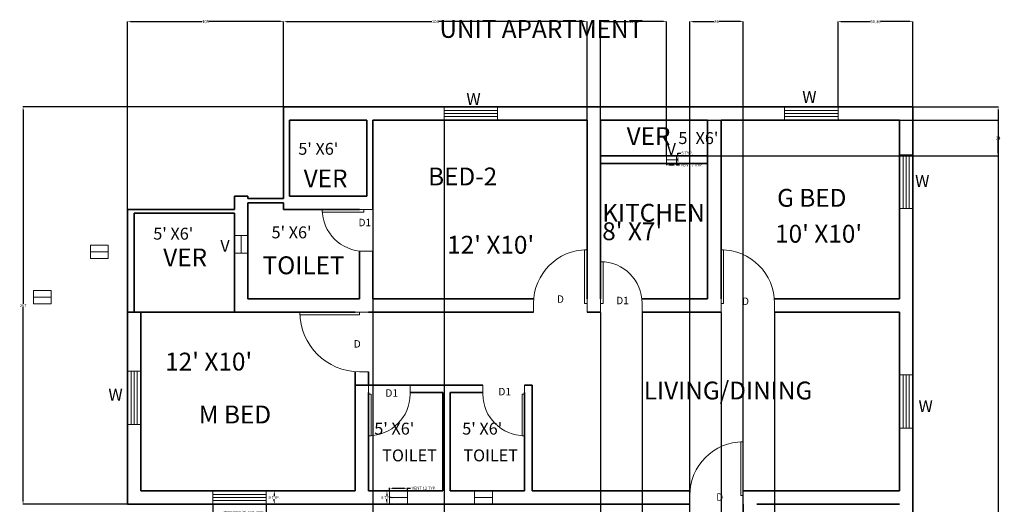
# Model space of a CAD drawing. Units: inches. Extents: x 168 to 831, y 504 to 1681.
# Tile 3 of 3: x 169 to 831, y 1355 to 1681. Entities that reach past the tile are written whole.
import ezdxf

# ---------------------------------------------------------------- set-up
doc = ezdxf.new("R2010")
doc.units = ezdxf.units.IN
doc.header["$MEASUREMENT"] = 0
for name, color, linetype, lineweight in [('A-ANNO-DIMS', 2, 'Continuous', 13), ('A-ANNO-TEXT', 7, 'Continuous', 18), ('A-AREA-IDEN', 7, 'Continuous', 18), ('A-DOOR', 3, 'Continuous', 18), ('A-GLAZ', 4, 'Continuous', 18), ('A-WALL', 7, 'Continuous', 35)]:
    doc.layers.add(name, color=color, linetype=linetype, lineweight=lineweight)
doc.styles.get("Standard").update_dxf_attribs({"font": 'arial.ttf'})
doc.dimstyles.get("Standard").update_dxf_attribs({"dimtxt": 2, "dimasz": 2, "dimexe": 0.18, "dimexo": 0.0625, "dimgap": 0.09, "dimtad": 0, "dimtih": 1, "dimtoh": 1, "dimdec": 0, "dimzin": 0, "dimdsep": 46, "dimlunit": 3, "dimtxsty": 'Standard', "dimcen": 0.09, "dimadec": 0, "dimazin": 0, "dimtfac": 1, "dimtdec": 0, "dimtofl": 0, "dimtmove": 0, "dimatfit": 3, "dimfxl": 1, "dimtolj": 1, "dimtzin": 0, "dimarcsym": 0})

# ---------------------------------------------------------------- blocks, each defined once
blk = doc.blocks.new('*U2')
for p, q in [((0, 0), (0, -6)), ((36, 0), (36, -6))]:
    blk.add_line(p, q)
blk.add_lwpolyline([(0, 0), (0, 36), (1.75, 36), (1.75, 0)], close=True)
blk.add_arc((0, 0), 36, 0, 90)
blk = doc.blocks.new('*U3')
for p, q in [((0, 0), (0, -6)), ((-36, 0), (-36, -6))]:
    blk.add_line(p, q)
blk.add_lwpolyline([(0, 0), (0, 36), (-1.75, 36), (-1.75, 0)], close=True)
blk.add_arc((0, 0), 36, 90, 180)
blk = doc.blocks.new('*U4')
for p, q in [((0, 0), (0, -6)), ((28, 0), (28, -6))]:
    blk.add_line(p, q)
blk.add_lwpolyline([(0, 0), (0, 28), (1.75, 28), (1.75, 0)], close=True)
blk.add_arc((0, 0), 28, 0, 90)
blk = doc.blocks.new('*U5')
for p, q in [((-28, 0), (-28, -6)), ((0, 0), (0, -6))]:
    blk.add_line(p, q)
blk.add_lwpolyline([(0, 0), (0, 28), (-1.75, 28), (-1.75, 0)], close=True)
blk.add_arc((0, 0), 28, 90, 180)
blk = doc.blocks.new('*U6')
for p, q in [((0, 0), (0, -6)), ((28, 0), (28, -6))]:
    blk.add_line(p, q)
blk.add_lwpolyline([(0, 0), (0, 28), (1.75, 28), (1.75, 0)], close=True)
blk.add_arc((0, 0), 28, 0, 90)
blk = doc.blocks.new('*U7')
for p, q in [((0, 0), (0, -6)), ((40, 0), (40, -6))]:
    blk.add_line(p, q)
blk.add_lwpolyline([(0, 0), (0, 40), (1.75, 40), (1.75, 0)], close=True)
blk.add_arc((0, 0), 40, 0, 90)
blk = doc.blocks.new('*U8')
for p, q in [((0, 0), (0, -6)), ((28, 0), (28, -6))]:
    blk.add_line(p, q)
blk.add_lwpolyline([(0, 0), (0, 28), (1.75, 28), (1.75, 0)], close=True)
blk.add_arc((0, 0), 28, 0, 90)
blk = doc.blocks.new('WIN-36IN')
for p, q in [((0, 6.5), (36, 6.5)), ((0, 4.5), (36, 4.5)), ((0, 2.5), (36, 2.5))]:
    blk.add_line(p, q)
blk.add_lwpolyline([(36, 0), (36, 9), (0, 9), (0, 0)], close=True)
blk = doc.blocks.new('VENT-12IN')
blk.add_line((0, 4.5), (12, 4.5))
blk.add_lwpolyline([(0, 0), (0, 9), (12, 9), (12, 0)], close=True)
blk = doc.blocks.new('VENT-KITCHEN-SMALL')
blk.add_line((0, 2.52), (6.62, 2.52))
blk.add_lwpolyline([(0, 0.03), (0, 5), (6.62, 5), (6.62, 0)], close=True)
blk = doc.blocks.new('*D20')
at = {"layer": 'A-ANNO-DIMS', "color": 0, "lineweight": -2, "transparency": 16777216}
for p, q in [((299.21, 1354.98), (299.21, 1349.46)), ((335.21, 1354.98), (335.21, 1349.46)), ((301.21, 1349.64), (305.7, 1349.64)), ((333.21, 1349.64), (328.73, 1349.64))]:
    blk.add_line(p, q, dxfattribs=at)
at = {"layer": 'A-ANNO-DIMS', "color": 0, "transparency": 16777216}
for points in [[(301.21, 1349.97), (301.21, 1349.31), (299.21, 1349.64)], [(333.21, 1349.97), (333.21, 1349.31), (335.21, 1349.64)]]:
    blk.add_solid(points, dxfattribs=at)
at = {"layer": 'Defpoints', "color": 0, "transparency": 16777216}
for p in [(299.21, 1355.04), (335.21, 1355.04), (335.21, 1349.64)]:
    blk.add_point(p, dxfattribs=at)
at = {"layer": 'A-ANNO-DIMS', "color": 0, "transparency": 16777216, "insert": (317.21, 1349.64), "char_height": 2, "attachment_point": 5}
blk.add_mtext('\\A1;WINDOW 36 TYP.', dxfattribs=at)
blk = doc.blocks.new('*D21')
at = {"layer": 'A-ANNO-DIMS', "color": 0, "lineweight": -2, "transparency": 16777216}
for p, q in [((335.28, 1364.04), (340.79, 1364.04)), ((340.61, 1362.04), (340.61, 1360.65)), ((340.61, 1357.04), (340.61, 1358.43)), ((335.28, 1355.04), (340.79, 1355.04))]:
    blk.add_line(p, q, dxfattribs=at)
at = {"layer": 'A-ANNO-DIMS', "color": 0, "transparency": 16777216}
for points in [[(340.28, 1362.04), (340.95, 1362.04), (340.61, 1364.04)], [(340.28, 1357.04), (340.95, 1357.04), (340.61, 1355.04)]]:
    blk.add_solid(points, dxfattribs=at)
at = {"layer": 'Defpoints', "color": 0, "transparency": 16777216}
for p in [(335.21, 1364.04), (340.61, 1364.04), (335.21, 1355.04)]:
    blk.add_point(p, dxfattribs=at)
at = {"layer": 'A-ANNO-DIMS', "color": 0, "transparency": 16777216, "insert": (340.61, 1359.54), "char_height": 2, "attachment_point": 5}
blk.add_mtext('\\A1;9 TYP.', dxfattribs=at)
blk = doc.blocks.new('*D22')
at = {"layer": 'A-ANNO-DIMS', "color": 0, "lineweight": -2, "transparency": 16777216}
for p, q in [((418.11, 1364.1), (418.11, 1366.02)), ((420.11, 1365.84), (428.11, 1365.84)), ((430.11, 1364.1), (430.11, 1366.02)), ((430.11, 1365.84), (432.11, 1365.84))]:
    blk.add_line(p, q, dxfattribs=at)
at = {"layer": 'A-ANNO-DIMS', "color": 0, "transparency": 16777216}
for points in [[(420.11, 1366.17), (420.11, 1365.51), (418.11, 1365.84)], [(428.11, 1366.17), (428.11, 1365.51), (430.11, 1365.84)]]:
    blk.add_solid(points, dxfattribs=at)
at = {"layer": 'Defpoints', "color": 0, "transparency": 16777216}
for p in [(418.11, 1364.04), (430.11, 1365.84), (430.11, 1364.04)]:
    blk.add_point(p, dxfattribs=at)
at = {"layer": 'A-ANNO-DIMS', "color": 0, "transparency": 16777216, "insert": (441.24, 1365.84), "char_height": 2, "attachment_point": 5}
blk.add_mtext('\\A1;VENT 12 TYP.', dxfattribs=at)
blk = doc.blocks.new('*D23')
at = {"layer": 'A-ANNO-DIMS', "color": 0, "lineweight": -2, "transparency": 16777216}
for p, q in [((418.05, 1364.04), (416.13, 1364.04)), ((416.31, 1362.04), (416.31, 1360.65)), ((416.31, 1357.04), (416.31, 1358.43)), ((418.05, 1355.04), (416.13, 1355.04))]:
    blk.add_line(p, q, dxfattribs=at)
at = {"layer": 'A-ANNO-DIMS', "color": 0, "transparency": 16777216}
for points in [[(415.98, 1362.04), (416.65, 1362.04), (416.31, 1364.04)], [(415.98, 1357.04), (416.65, 1357.04), (416.31, 1355.04)]]:
    blk.add_solid(points, dxfattribs=at)
at = {"layer": 'Defpoints', "color": 0, "transparency": 16777216}
for p in [(416.31, 1364.04), (418.11, 1364.04), (418.11, 1355.04)]:
    blk.add_point(p, dxfattribs=at)
at = {"layer": 'A-ANNO-DIMS', "color": 0, "transparency": 16777216, "insert": (416.31, 1359.54), "char_height": 2, "attachment_point": 5}
blk.add_mtext('\\A1;9 TYP.', dxfattribs=at)
blk = doc.blocks.new('*D24')
at = {"layer": 'A-ANNO-DIMS', "color": 0, "lineweight": -2, "transparency": 16777216}
for p, q in [((604.31, 1583.98), (604.31, 1582.87)), ((606.31, 1583.05), (608.93, 1583.05)), ((610.93, 1583.98), (610.93, 1582.87)), ((610.93, 1583.05), (612.93, 1583.05))]:
    blk.add_line(p, q, dxfattribs=at)
at = {"layer": 'A-ANNO-DIMS', "color": 0, "transparency": 16777216}
for points in [[(606.31, 1583.38), (606.31, 1582.71), (604.31, 1583.05)], [(608.93, 1583.38), (608.93, 1582.71), (610.93, 1583.05)]]:
    blk.add_solid(points, dxfattribs=at)
at = {"layer": 'Defpoints', "color": 0, "transparency": 16777216}
for p in [(604.31, 1584.04), (610.93, 1584.04), (610.93, 1583.05)]:
    blk.add_point(p, dxfattribs=at)
at = {"layer": 'A-ANNO-DIMS', "color": 0, "transparency": 16777216, "insert": (621.27, 1583.05), "char_height": 2, "attachment_point": 5}
blk.add_mtext('\\A1;VENT 7 TYP.', dxfattribs=at)
blk = doc.blocks.new('*D25')
at = {"layer": 'A-ANNO-DIMS', "color": 0, "lineweight": -2, "transparency": 16777216}
for p, q in [((610.99, 1589.04), (612.1, 1589.04)), ((611.92, 1589.04), (611.92, 1591.04)), ((611.92, 1591.04), (613.92, 1591.04)), ((610.99, 1584.04), (612.1, 1584.04)), ((611.92, 1586.04), (611.92, 1587.04))]:
    blk.add_line(p, q, dxfattribs=at)
at = {"layer": 'A-ANNO-DIMS', "color": 0, "transparency": 16777216}
for points in [[(611.59, 1587.04), (612.25, 1587.04), (611.92, 1589.04)], [(611.59, 1586.04), (612.25, 1586.04), (611.92, 1584.04)]]:
    blk.add_solid(points, dxfattribs=at)
at = {"layer": 'Defpoints', "color": 0, "transparency": 16777216}
for p in [(610.93, 1589.04), (611.92, 1589.04), (610.93, 1584.04)]:
    blk.add_point(p, dxfattribs=at)
at = {"layer": 'A-ANNO-DIMS', "color": 0, "transparency": 16777216, "insert": (618.1, 1591.04), "char_height": 2, "attachment_point": 5}
blk.add_mtext('\\A1;5 TYP.', dxfattribs=at)
blk = doc.blocks.new('*D31')
at = {"layer": 'A-ANNO-DIMS', "color": 0, "lineweight": -2, "transparency": 16777216}
for p, q in [((769.93, 1622.04), (827.29, 1622.04)), ((827.11, 1620.04), (827.11, 1093.58)), ((827.11, 564.91), (827.11, 1091.36)), ((769.93, 562.91), (827.29, 562.91))]:
    blk.add_line(p, q, dxfattribs=at)
at = {"layer": 'A-ANNO-DIMS', "color": 0, "transparency": 16777216}
for points in [[(826.78, 1620.04), (827.45, 1620.04), (827.11, 1622.04)], [(826.78, 564.91), (827.45, 564.91), (827.11, 562.91)]]:
    blk.add_solid(points, dxfattribs=at)
at = {"layer": 'Defpoints', "color": 0, "transparency": 16777216}
for p in [(769.86, 1622.04), (827.11, 1622.04), (769.86, 562.91)]:
    blk.add_point(p, dxfattribs=at)
at = {"layer": 'A-ANNO-DIMS', "color": 0, "transparency": 16777216, "insert": (827.11, 1092.47), "char_height": 2, "attachment_point": 5}
blk.add_mtext('\\A1;1059.1', dxfattribs=at)
blk = doc.blocks.new('*D36')
at = {"layer": 'A-ANNO-DIMS', "color": 0, "lineweight": -2, "transparency": 16777216}
for p, q in [((346.8, 1622.04), (171.56, 1622.04)), ((171.74, 1620.04), (171.74, 1489.65)), ((171.74, 1357.04), (171.74, 1487.43)), ((241.8, 1355.04), (171.56, 1355.04))]:
    blk.add_line(p, q, dxfattribs=at)
at = {"layer": 'A-ANNO-DIMS', "color": 0, "transparency": 16777216}
for points in [[(171.41, 1620.04), (172.08, 1620.04), (171.74, 1622.04)], [(171.41, 1357.04), (172.08, 1357.04), (171.74, 1355.04)]]:
    blk.add_solid(points, dxfattribs=at)
at = {"layer": 'Defpoints', "color": 0, "transparency": 16777216}
for p in [(171.74, 1622.04), (346.86, 1622.04), (241.86, 1355.04)]:
    blk.add_point(p, dxfattribs=at)
at = {"layer": 'A-ANNO-DIMS', "color": 0, "transparency": 16777216, "insert": (171.74, 1488.54), "char_height": 2, "attachment_point": 5}
blk.add_mtext('\\A1;267', dxfattribs=at)
blk = doc.blocks.new('*D37')
at = {"layer": 'A-ANNO-DIMS', "color": 0, "lineweight": -2, "transparency": 16777216}
for p, q in [((241.86, 1553.1), (241.86, 1679.47)), ((243.86, 1679.29), (292.15, 1679.29)), ((344.86, 1679.29), (296.58, 1679.29)), ((346.86, 1622.1), (346.86, 1679.47))]:
    blk.add_line(p, q, dxfattribs=at)
at = {"layer": 'A-ANNO-DIMS', "color": 0, "transparency": 16777216}
for points in [[(243.86, 1679.62), (243.86, 1678.96), (241.86, 1679.29)], [(344.86, 1679.62), (344.86, 1678.96), (346.86, 1679.29)]]:
    blk.add_solid(points, dxfattribs=at)
at = {"layer": 'Defpoints', "color": 0, "transparency": 16777216}
for p in [(346.86, 1679.29), (346.86, 1622.04), (241.86, 1553.04)]:
    blk.add_point(p, dxfattribs=at)
at = {"layer": 'A-ANNO-DIMS', "color": 0, "transparency": 16777216, "insert": (294.36, 1679.29), "char_height": 2, "attachment_point": 5}
blk.add_mtext('\\A1;105', dxfattribs=at)
blk = doc.blocks.new('*D38')
at = {"layer": 'A-ANNO-DIMS', "color": 0, "lineweight": -2, "transparency": 16777216}
for p, q in [((346.86, 1622.1), (346.86, 1679.47)), ((348.86, 1679.29), (446.55, 1679.29)), ((548.86, 1679.29), (451.18, 1679.29)), ((550.86, 1613.1), (550.86, 1679.47))]:
    blk.add_line(p, q, dxfattribs=at)
at = {"layer": 'A-ANNO-DIMS', "color": 0, "transparency": 16777216}
for points in [[(348.86, 1679.62), (348.86, 1678.96), (346.86, 1679.29)], [(548.86, 1679.62), (548.86, 1678.96), (550.86, 1679.29)]]:
    blk.add_solid(points, dxfattribs=at)
at = {"layer": 'Defpoints', "color": 0, "transparency": 16777216}
for p in [(550.86, 1679.29), (346.86, 1622.04), (550.86, 1613.04)]:
    blk.add_point(p, dxfattribs=at)
at = {"layer": 'A-ANNO-DIMS', "color": 0, "transparency": 16777216, "insert": (448.86, 1679.29), "char_height": 2, "attachment_point": 5}
blk.add_mtext('\\A1;204', dxfattribs=at)
blk = doc.blocks.new('*D40')
at = {"layer": 'A-ANNO-DIMS', "color": 0, "lineweight": -2, "transparency": 16777216}
for p, q in [((619.86, 902.1), (619.86, 1679.47)), ((621.86, 1679.29), (636.34, 1679.29)), ((653.86, 1679.29), (639.38, 1679.29)), ((655.86, 946.97), (655.86, 1679.47))]:
    blk.add_line(p, q, dxfattribs=at)
at = {"layer": 'A-ANNO-DIMS', "color": 0, "transparency": 16777216}
for points in [[(621.86, 1679.62), (621.86, 1678.96), (619.86, 1679.29)], [(653.86, 1679.62), (653.86, 1678.96), (655.86, 1679.29)]]:
    blk.add_solid(points, dxfattribs=at)
at = {"layer": 'Defpoints', "color": 0, "transparency": 16777216}
for p in [(655.86, 1679.29), (655.86, 946.91), (619.86, 902.04)]:
    blk.add_point(p, dxfattribs=at)
at = {"layer": 'A-ANNO-DIMS', "color": 0, "transparency": 16777216, "insert": (637.86, 1679.29), "char_height": 2, "attachment_point": 5}
blk.add_mtext('\\A1;36', dxfattribs=at)
blk = doc.blocks.new('*D47')
at = {"layer": 'A-ANNO-DIMS', "color": 0, "lineweight": -2, "transparency": 16777216}
for p, q in [((559.86, 1483.98), (559.86, 505.48)), ((587.86, 1483.98), (587.86, 505.48)), ((561.86, 505.66), (572.32, 505.66)), ((585.86, 505.66), (575.4, 505.66))]:
    blk.add_line(p, q, dxfattribs=at)
at = {"layer": 'A-ANNO-DIMS', "color": 0, "transparency": 16777216}
for points in [[(561.86, 505.99), (561.86, 505.32), (559.86, 505.66)], [(585.86, 505.99), (585.86, 505.32), (587.86, 505.66)]]:
    blk.add_solid(points, dxfattribs=at)
at = {"layer": 'Defpoints', "color": 0, "transparency": 16777216}
for p in [(559.86, 1484.04), (587.86, 1484.04), (587.86, 505.66)]:
    blk.add_point(p, dxfattribs=at)
at = {"layer": 'A-ANNO-DIMS', "color": 0, "transparency": 16777216, "insert": (573.86, 505.66), "char_height": 2, "attachment_point": 5}
blk.add_mtext('\\A1;28', dxfattribs=at)
blk = doc.blocks.new('*D48')
at = {"layer": 'A-ANNO-DIMS', "color": 0, "lineweight": -2, "transparency": 16777216}
for p, q in [((640.86, 1483.98), (640.86, 505.48)), ((676.86, 1483.98), (676.86, 505.48)), ((642.86, 505.66), (657.34, 505.66)), ((674.86, 505.66), (660.38, 505.66))]:
    blk.add_line(p, q, dxfattribs=at)
at = {"layer": 'A-ANNO-DIMS', "color": 0, "transparency": 16777216}
for points in [[(642.86, 505.99), (642.86, 505.32), (640.86, 505.66)], [(674.86, 505.99), (674.86, 505.32), (676.86, 505.66)]]:
    blk.add_solid(points, dxfattribs=at)
at = {"layer": 'Defpoints', "color": 0, "transparency": 16777216}
for p in [(640.86, 1484.04), (676.86, 1484.04), (676.86, 505.66)]:
    blk.add_point(p, dxfattribs=at)
at = {"layer": 'A-ANNO-DIMS', "color": 0, "transparency": 16777216, "insert": (658.86, 505.66), "char_height": 2, "attachment_point": 5}
blk.add_mtext('\\A1;36', dxfattribs=at)
blk = doc.blocks.new('*D49')
at = {"layer": 'A-ANNO-DIMS', "color": 0, "lineweight": -2, "transparency": 16777216}
for p, q in [((559.86, 1589.1), (559.86, 1679.47)), ((561.86, 1679.29), (578.58, 1679.29)), ((602.31, 1679.29), (585.58, 1679.29)), ((604.31, 1589.1), (604.31, 1679.47))]:
    blk.add_line(p, q, dxfattribs=at)
at = {"layer": 'A-ANNO-DIMS', "color": 0, "transparency": 16777216}
for points in [[(561.86, 1679.62), (561.86, 1678.96), (559.86, 1679.29)], [(602.31, 1679.62), (602.31, 1678.96), (604.31, 1679.29)]]:
    blk.add_solid(points, dxfattribs=at)
at = {"layer": 'Defpoints', "color": 0, "transparency": 16777216}
for p in [(604.31, 1679.29), (559.86, 1589.04), (604.31, 1589.04)]:
    blk.add_point(p, dxfattribs=at)
at = {"layer": 'A-ANNO-DIMS', "color": 0, "transparency": 16777216, "insert": (582.08, 1679.29), "char_height": 2, "attachment_point": 5}
blk.add_mtext('\\A1;44.44', dxfattribs=at)
blk = doc.blocks.new('*D50')
at = {"layer": 'A-ANNO-DIMS', "color": 0, "lineweight": -2, "transparency": 16777216}
for p, q in [((631.93, 1613.04), (827.29, 1613.04)), ((827.11, 1611.04), (827.11, 1602.13)), ((827.11, 1591.04), (827.11, 1599.94)), ((631.93, 1589.04), (827.29, 1589.04))]:
    blk.add_line(p, q, dxfattribs=at)
at = {"layer": 'A-ANNO-DIMS', "color": 0, "transparency": 16777216}
for points in [[(826.78, 1611.04), (827.45, 1611.04), (827.11, 1613.04)], [(826.78, 1591.04), (827.45, 1591.04), (827.11, 1589.04)]]:
    blk.add_solid(points, dxfattribs=at)
at = {"layer": 'Defpoints', "color": 0, "transparency": 16777216}
for p in [(631.86, 1613.04), (827.11, 1613.04), (631.86, 1589.04)]:
    blk.add_point(p, dxfattribs=at)
at = {"layer": 'A-ANNO-DIMS', "color": 0, "transparency": 16777216, "insert": (827.11, 1601.04), "char_height": 2, "attachment_point": 5}
blk.add_mtext('\\A1;24', dxfattribs=at)
blk = doc.blocks.new('*D51')
at = {"layer": 'A-ANNO-DIMS', "color": 0, "lineweight": -2, "transparency": 16777216}
for p, q in [((719.5, 1622.1), (719.5, 1679.47)), ((721.5, 1679.29), (741.22, 1679.29)), ((767.86, 1679.29), (748.15, 1679.29)), ((769.86, 1622.1), (769.86, 1679.47))]:
    blk.add_line(p, q, dxfattribs=at)
at = {"layer": 'A-ANNO-DIMS', "color": 0, "transparency": 16777216}
for points in [[(721.5, 1679.62), (721.5, 1678.96), (719.5, 1679.29)], [(767.86, 1679.62), (767.86, 1678.96), (769.86, 1679.29)]]:
    blk.add_solid(points, dxfattribs=at)
at = {"layer": 'Defpoints', "color": 0, "transparency": 16777216}
for p in [(769.86, 1679.29), (719.5, 1622.04), (769.86, 1622.04)]:
    blk.add_point(p, dxfattribs=at)
at = {"layer": 'A-ANNO-DIMS', "color": 0, "transparency": 16777216, "insert": (744.68, 1679.29), "char_height": 2, "attachment_point": 5}
blk.add_mtext('\\A1;50.36', dxfattribs=at)
blk = doc.blocks.new('*D52')
at = {"layer": 'A-ANNO-DIMS', "color": 0, "lineweight": -2, "transparency": 16777216}
for p, q in [((406.86, 1612.98), (406.86, 505.48)), ((454.72, 1612.98), (454.72, 505.48)), ((408.86, 505.66), (427.29, 505.66)), ((452.72, 505.66), (434.3, 505.66))]:
    blk.add_line(p, q, dxfattribs=at)
at = {"layer": 'A-ANNO-DIMS', "color": 0, "transparency": 16777216}
for points in [[(408.86, 505.99), (408.86, 505.32), (406.86, 505.66)], [(452.72, 505.99), (452.72, 505.32), (454.72, 505.66)]]:
    blk.add_solid(points, dxfattribs=at)
at = {"layer": 'Defpoints', "color": 0, "transparency": 16777216}
for p in [(406.86, 1613.04), (454.72, 1613.04), (454.72, 505.66)]:
    blk.add_point(p, dxfattribs=at)
at = {"layer": 'A-ANNO-DIMS', "color": 0, "transparency": 16777216, "insert": (430.79, 505.66), "char_height": 2, "attachment_point": 5}
blk.add_mtext('\\A1;47.86', dxfattribs=at)

msp = doc.modelspace()

# ---------------------------------------------------------------- linework, layer by layer
at = {"layer": 'A-WALL'}
for p, q in [((346.863, 1622.039), (769.863, 1622.039)), ((346.863, 1562.039), (346.863, 1622.039)), ((769.863, 1622.039), (769.863, 1197.039)), ((350.863, 1613.039), (402.863, 1613.039)), ((350.863, 1562.039), (350.863, 1613.039)), ((402.863, 1562.039), (402.863, 1613.039)), ((406.863, 1613.039), (550.863, 1613.039)), ((406.863, 1553.039), (406.863, 1613.039)), ((550.863, 1613.039), (550.863, 1493.039)), ((559.863, 1613.039), (559.863, 1493.039)), ((559.863, 1582.039), (559.863, 1613.039)), ((559.863, 1613.039), (631.863, 1613.039)), ((631.863, 1613.039), (631.863, 1493.039)), ((640.863, 1613.039), (640.863, 1493.039)), ((640.863, 1613.039), (760.863, 1613.039)), ((760.863, 1613.039), (760.863, 1493.039)), ((631.863, 1589.039), (559.863, 1589.039)), ((631.863, 1584.039), (559.863, 1584.039)), ((322.863, 1562.039), (313.863, 1562.039)), ((313.863, 1553.039), (313.863, 1562.039)), ((322.863, 1560.539), (322.863, 1562.039)), ((346.863, 1562.039), (346.863, 1560.539)), ((402.863, 1562.039), (350.863, 1562.039)), ((346.863, 1560.539), (322.863, 1560.539)), ((322.863, 1493.039), (322.863, 1557.539)), ((346.863, 1557.539), (322.863, 1557.539)), ((346.863, 1557.539), (346.863, 1557.539)), ((346.863, 1557.539), (346.863, 1553.039)), ((241.863, 1484.039), (241.863, 1553.039)), ((313.863, 1553.039), (241.863, 1553.039)), ((313.863, 1550.539), (246.363, 1550.539)), ((246.363, 1484.039), (246.363, 1550.539)), ((313.863, 1548.039), (313.863, 1550.539)), ((397.863, 1553.039), (346.863, 1553.039)), ((313.863, 1484.039), (313.863, 1548.039)), ((397.863, 1493.039), (397.863, 1525.2)), ((406.863, 1493.039), (406.863, 1525.039)), ((397.863, 1493.039), (322.863, 1493.039)), ((514.989, 1493.039), (406.863, 1493.039)), ((631.863, 1493.039), (587.702, 1493.039)), ((640.863, 1493.039), (640.863, 1493.039)), ((760.863, 1493.039), (676.863, 1493.039)), ((241.863, 1484.039), (394.863, 1484.039)), ((241.863, 1355.039), (241.863, 1484.039)), ((250.863, 1484.039), (394.863, 1484.039)), ((250.863, 1484.039), (394.863, 1484.039)), ((250.863, 1364.039), (250.863, 1484.039)), ((250.863, 1364.039), (250.863, 1484.039)), ((403.863, 1484.039), (514.863, 1484.039)), ((550.863, 1484.039), (559.863, 1484.039)), ((587.863, 1484.039), (640.863, 1484.039)), ((676.863, 1484.039), (760.863, 1484.039)), ((760.863, 1484.039), (760.863, 1364.039)), ((394.863, 1444.151), (394.863, 1364.039)), ((403.863, 1444.039), (403.863, 1435.039)), ((458.863, 1435.039), (394.863, 1435.039)), ((403.863, 1430.039), (403.863, 1364.039)), ((403.863, 1430.039), (403.863, 1364.039)), ((453.863, 1430.039), (431.863, 1430.039)), ((453.863, 1364.039), (453.863, 1430.039)), ((480.863, 1435.039), (458.863, 1435.039)), ((458.863, 1364.039), (458.863, 1430.039)), ((480.863, 1430.039), (458.863, 1430.039)), ((458.863, 1430.039), (458.863, 1364.039)), ((513.863, 1435.039), (508.863, 1435.039)), ((508.863, 1364.039), (508.863, 1430.039)), ((513.863, 1364.039), (513.863, 1435.039)), ((769.863, 1406.112), (769.863, 979.3)), ((394.863, 1364.039), (250.863, 1364.039)), ((453.863, 1364.039), (403.863, 1364.039)), ((508.863, 1364.039), (458.863, 1364.039)), ((619.863, 1364.039), (513.863, 1364.039)), ((760.863, 1364.039), (655.863, 1364.039)), ((241.863, 1355.039), (619.863, 1355.039)), ((655.863, 1355.039), (655.863, 1197.039)), ((664.863, 1355.039), (760.863, 1355.039))]:
    msp.add_line(p, q, dxfattribs=at)

# ---------------------------------------------------------------- block references
at = {"layer": 'A-DOOR', "xscale": -1}
for name, p, rotation in [('*U8', (400.863, 1553.039), 90), ('*U7', (397.863, 1484.039), 90), ('*U6', (403.863, 1429.039), 180), ('*U5', (508.863, 1429.039), 180)]:
    msp.add_blockref(name, p, dxfattribs=dict(at, rotation=rotation))
msp.add_blockref('*U2', (550.863, 1490.039), dxfattribs=at)
at = {"layer": 'A-DOOR'}
for name, p in [('*U2', (640.863, 1490.039)), ('*U4', (559.863, 1490.039)), ('*U3', (655.863, 1361.039))]:
    msp.add_blockref(name, p, dxfattribs=at)
at = {"layer": 'A-GLAZ'}
for name, p in [('WIN-36IN', (454.72, 1613.039)), ('WIN-36IN', (683.502, 1613.039)), ('VENT-KITCHEN-SMALL', (604.305, 1584.039)), ('VENT-12IN', (216.994, 1520.204)), ('VENT-12IN', (178.643, 1489.617)), ('WIN-36IN', (299.212, 1355.039)), ('WIN-36IN', (299.212, 1355.039)), ('VENT-12IN', (418.112, 1355.039)), ('VENT-12IN', (475.211, 1355.039))]:
    msp.add_blockref(name, p, dxfattribs=at)
for name, p, rotation in [('WIN-36IN', (760.864, 1589.849), 270.0000000000011), ('VENT-12IN', (322.863, 1523.695), 89.9999999999985), ('WIN-36IN', (241.864, 1444.544), 270.0000000000007), ('WIN-36IN', (760.864, 1442.112), 270.0000000000007)]:
    msp.add_blockref(name, p, dxfattribs=dict(at, rotation=rotation))

# ---------------------------------------------------------------- texts
at = {"layer": 'A-ANNO-DIMS', "attachment_point": 1}
for s, width, insert, char_height in [("5' X6'", 59.10581, (612.206, 1605.06), 8), ("5' X6'", 59.10581, (356.741, 1597.861), 8), ("5' X6'", 59.10581, (338.758, 1541.708), 8), ("8' X7'", 157.93148, (561.014, 1544.48), 12), ("10' X10'", 157.93148, (677.207, 1542.818), 12), ("5' X6'", 59.10581, (259.258, 1540.831), 8), ("12' X10'", 157.93148, (456.793, 1535.408), 12), ("12' X10'", 157.93148, (267.254, 1456.911), 12), ("5' X6'", 59.10581, (407.825, 1409.864), 8), ("5' X6'", 59.10581, (466.931, 1409.864), 8)]:
    msp.add_mtext_dynamic_manual_height_columns(s, width=width, gutter_width=1, heights=[0], dxfattribs=dict(at, insert=insert, char_height=char_height))
at = {"layer": 'A-ANNO-TEXT', "attachment_point": 1}
for s, width, insert, char_height in [('UNIT APARTMENT', 581.57412, (451.609, 1680.396), 12), ('W', 57.92772, (469.717, 1631.288), 8), ('W', 57.92772, (695.469, 1632.7), 8), ('V', 20.00841, (604.274, 1597.733), 8), ('V', 20.00841, (604.274, 1597.733), 8), ('W', 57.92772, (771.346, 1576.224), 8), ('D1', 11.24528, (397.209, 1546.839), 5), ('V', 20.00841, (304.33, 1532.662), 8), ('D', 11.24528, (530.576, 1495.405), 5), ('D1', 11.24528, (570.425, 1494.434), 5), ('D', 11.24528, (654.982, 1493.949), 5), ('D', 11.24528, (394.021, 1465.311), 5), ('W', 57.92772, (229.118, 1432.648), 8), ('D1', 11.24528, (415.277, 1432.303), 5), ('D1', 11.24528, (491.256, 1433.235), 5), ('W', 57.92772, (773.62, 1424.95), 8), ('D', 11.24528, (637.616, 1362.383), 5)]:
    msp.add_mtext_dynamic_manual_height_columns(s, width=width, gutter_width=1, heights=[0], dxfattribs=dict(at, insert=insert, char_height=char_height))
at = {"layer": 'A-AREA-IDEN', "attachment_point": 1}
for s, insert, char_height in [('VER', (577.442, 1608.367), 12), ('VER', (360.361, 1579.924), 12), ('BED-2', (443.993, 1581.273), 12), ('G BED', (678.553, 1566.92), 12), ('KITCHEN', (561.014, 1556.889), 12), ('VER', (265.944, 1526.857), 12), ('TOILET', (332.756, 1521.606), 12), ('LIVING/DINING', (588.938, 1437.474), 12), ('M BED', (289.837, 1421.362), 12), ('TOILET', (413.129, 1391.886), 8), ('TOILET', (467.672, 1391.886), 8)]:
    msp.add_mtext_dynamic_manual_height_columns(s, width=54.54242, gutter_width=1, heights=[0], dxfattribs=dict(at, insert=insert, char_height=char_height))

# ---------------------------------------------------------------- dimensions: what is measured, and where the dimension line sits
at = {"layer": 'A-ANNO-DIMS'}
for base, p1, p2, override, picture, middle in [((346.863, 1679.289), (241.863, 1553.039), (346.863, 1622.039), {"dimdec": 0, "dimlfac": 1, "dimrnd": 0, "dimzin": 0, "dimdsep": 46, "dimlunit": 2}, '*D37', (294.363, 1679.289)), ((550.863, 1679.289), (346.863, 1622.039), (550.863, 1613.039), {"dimdec": 0, "dimlfac": 1, "dimrnd": 0, "dimzin": 0, "dimdsep": 46, "dimlunit": 2}, '*D38', (448.863, 1679.289)), ((604.305, 1679.289), (559.863, 1589.039), (604.305, 1589.039), {"dimdec": 2, "dimlfac": 1, "dimrnd": 0, "dimzin": 0, "dimdsep": 46, "dimlunit": 2}, '*D49', (582.084, 1679.289)), ((655.863, 1679.289), (619.863, 902.039), (655.863, 946.908), {"dimdec": 0, "dimlfac": 1, "dimrnd": 0, "dimzin": 0, "dimdsep": 46, "dimlunit": 2}, '*D40', (637.863, 1679.289)), ((769.863, 1679.289), (719.502, 1622.039), (769.863, 1622.039), {"dimdec": 2, "dimlfac": 1, "dimrnd": 0, "dimzin": 0, "dimdsep": 46, "dimlunit": 2}, '*D51', (744.683, 1679.289)), ((454.72, 505.658), (406.863, 1613.039), (454.72, 1613.039), {"dimdec": 2, "dimlfac": 1, "dimrnd": 0, "dimzin": 0, "dimdsep": 46, "dimlunit": 2}, '*D52', (430.792, 505.658)), ((587.863, 505.658), (559.863, 1484.039), (587.863, 1484.039), {"dimdec": 0, "dimlfac": 1, "dimrnd": 0, "dimzin": 0, "dimdsep": 46, "dimlunit": 2}, '*D47', (573.863, 505.658)), ((676.863, 505.658), (640.863, 1484.039), (676.863, 1484.039), {"dimdec": 0, "dimlfac": 1, "dimrnd": 0, "dimzin": 0, "dimdsep": 46, "dimlunit": 2}, '*D48', (658.863, 505.658))]:
    dim = msp.add_linear_dim(base=base, p1=p1, p2=p2, dimstyle='Standard', override=override, dxfattribs=at)
    dim.commit()
    dim.dimension.update_dxf_attribs({"geometry": picture, "text_midpoint": middle})
for base, p1, p2, override, picture, middle in [((171.744, 1622.039), (241.863, 1355.039), (346.863, 1622.039), {"dimdec": 0, "dimlfac": 1, "dimrnd": 0, "dimzin": 0, "dimdsep": 46, "dimlunit": 2}, '*D36', (171.744, 1488.539)), ((827.113, 1622.039), (769.863, 562.908), (769.863, 1622.039), {"dimdec": 1, "dimlfac": 1, "dimrnd": 0, "dimzin": 0, "dimdsep": 46, "dimlunit": 2}, '*D31', (827.113, 1092.474)), ((827.113, 1613.039), (631.863, 1589.039), (631.863, 1613.039), {"dimdec": 0, "dimlfac": 1, "dimrnd": 0, "dimzin": 0, "dimdsep": 46, "dimlunit": 2}, '*D50', (827.113, 1601.039))]:
    dim = msp.add_linear_dim(base=base, p1=p1, p2=p2, angle=90, dimstyle='Standard', override=override, dxfattribs=at)
    dim.commit()
    dim.dimension.update_dxf_attribs({"geometry": picture, "text_midpoint": middle})
for base, p1, p2, picture, middle in [((611.92, 1589.039), (610.927, 1584.039), (610.927, 1589.039), '*D25', (618.101, 1591.039)), ((340.613, 1364.039), (335.213, 1355.039), (335.213, 1364.039), '*D21', (340.613, 1359.539)), ((416.312, 1364.039), (418.112, 1355.039), (418.112, 1364.039), '*D23', (416.312, 1359.539))]:
    dim = msp.add_linear_dim(base=base, p1=p1, p2=p2, angle=90, text='<> TYP.', dimstyle='Standard', override={"dimdec": 0, "dimlfac": 1, "dimrnd": 0, "dimzin": 0, "dimdsep": 46, "dimlunit": 2}, dxfattribs=at)
    dim.commit()
    dim.dimension.update_dxf_attribs({"geometry": picture, "text_midpoint": middle})
for base, p1, p2, text, picture, middle in [((610.927, 1583.046), (604.305, 1584.039), (610.927, 1584.039), 'VENT <> TYP.', '*D24', (621.273, 1583.046)), ((430.112, 1365.839), (418.112, 1364.039), (430.112, 1364.039), 'VENT <> TYP.', '*D22', (441.235, 1365.839)), ((335.213, 1349.639), (299.213, 1355.039), (335.213, 1355.039), 'WINDOW <> TYP.', '*D20', (317.213, 1349.639))]:
    dim = msp.add_linear_dim(base=base, p1=p1, p2=p2, text=text, dimstyle='Standard', override={"dimdec": 0, "dimlfac": 1, "dimrnd": 0, "dimzin": 0, "dimdsep": 46, "dimlunit": 2}, dxfattribs=at)
    dim.commit()
    dim.dimension.update_dxf_attribs({"geometry": picture, "text_midpoint": middle})

doc.saveas('drawing.dxf')
